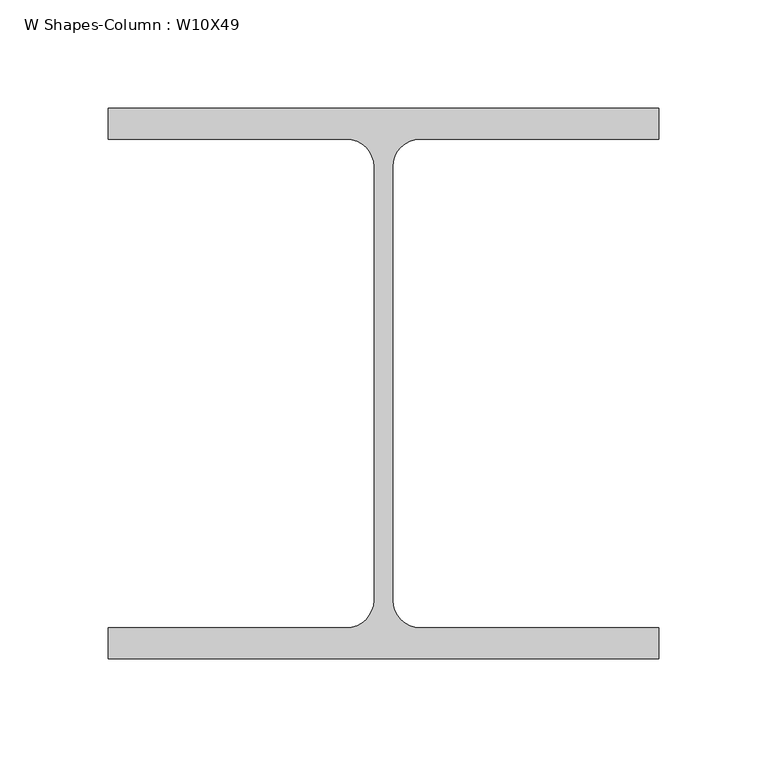
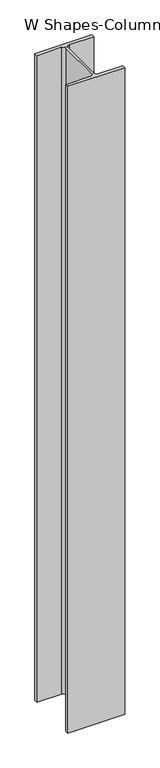
"""IFC4 building model written with IfcOpenShell, lengths in millimetres: column geometry, W Shapes-Column : W10X49."""

from ifc_helpers import new_model, si_unit, point, frame, frame_2d, origin, place, context, project, spatial, polyline, circle_curve, trimmed, segment, composite_curve, outline, extrude, source, transform, mapped, element, save


def w_shapes_column_w10x49_8035b166(model_context):
    return source(origin(), model_context, "Body", "SweptSolid", [
        extrude(outline(composite_curve([segment(polyline([(127.0, 127.0), (127.0, 112.776), (17.018, 112.776)]), True, "CONTINUOUS"), segment(trimmed(circle_curve(frame_2d((17.018, 100.076)), 12.7), [point((17.018, 112.776))], [point((4.318, 100.076))], True, "CARTESIAN"), True, "CONTINUOUS"), segment(polyline([(4.318, 100.076), (4.318, -100.076)]), True, "CONTINUOUS"), segment(trimmed(circle_curve(frame_2d((17.018, -100.076)), 12.7), [point((4.318, -100.076))], [point((17.018, -112.776))], True, "CARTESIAN"), True, "CONTINUOUS"), segment(polyline([(17.018, -112.776), (127.0, -112.776), (127.0, -127.0), (-127.0, -127.0), (-127.0, -112.776), (-17.018, -112.776)]), True, "CONTINUOUS"), segment(trimmed(circle_curve(frame_2d((-17.018, -100.076)), 12.7), [point((-17.018, -112.776))], [point((-4.318, -100.076))], True, "CARTESIAN"), True, "CONTINUOUS"), segment(polyline([(-4.318, -100.076), (-4.318, 100.076)]), True, "CONTINUOUS"), segment(trimmed(circle_curve(frame_2d((-17.018, 100.076)), 12.7), [point((-4.318, 100.076))], [point((-17.018, 112.776))], True, "CARTESIAN"), True, "CONTINUOUS"), segment(polyline([(-17.018, 112.776), (-127.0, 112.776), (-127.0, 127.0), (127.0, 127.0)]), True, "CONTINUOUS")], self_intersect=False)), frame((0.0, 0.0, 9144.0), z_axis=(0.0, 0.0, 1.0), x_axis=(1.0, 0.0, 0.0)), (0.0, 0.0, 1.0), 3048.0),
    ])


if __name__ == "__main__":
    model = new_model("IFC4")
    model_context = context("Model", 3, world=origin())
    ifc_project = project(units=[si_unit("LENGTHUNIT", "METRE", prefix="MILLI")], contexts=[model_context])
    site = spatial("IfcSite", under=ifc_project)
    building = spatial("IfcBuilding", under=site)
    placement = place(None, origin())
    w_shapes_column_w10x49_shape = w_shapes_column_w10x49_8035b166(model_context)
    element("IfcColumn", 1, ObjectType="W Shapes-Column : W10X49", at=placement, inside=building, context=model_context, shape_type="MappedRepresentation", body=[
        mapped(w_shapes_column_w10x49_shape, transform((0.0, 0.0, 0.0), x_axis=(1.0, 0.0, 0.0), y_axis=(0.0, 1.0, 0.0), z_axis=(0.0, 0.0, 1.0))),
    ])
    save(model, "model.ifc")

# Revit data of these elements
# Type "W Shapes-Column : W10X49"
#   Section Name Key = "W10x49"
#   Assembly Code = "B10"
#   Width = 10.000"
#   Web Thickness = 0.340"
#   Web Fillet = 0.500"
#   Warping Constant = 2070.00 in⁶
#   Torsional Moment of Inertia = 1.39 in⁴
#   Section Area = 14.40 in²
#   Plastic Modulus weak axis = 28.30 in³
#   Plastic Modulus strong axis = 60.40 in³
#   Perimeter = 58.50 ft²/ft
#   Nominal Weight = 49.00 lbf/ft
#   Moment of Inertia weak axis = 93.40 in⁴
#   Moment of Inertia strong axis = 272.00 in⁴
#   Height = 10.000"
#   Flange Thickness = 0.560"
#   Elastic Modulus weak axis = 18.70 in³
#   Elastic Modulus strong axis = 54.60 in³
#   Centroid Vertical = 5.000"
#   Centroid Horizontal = 5.000"
#   Bolt Spacing = 0' - 5 1/2"
#   Structural Material [instance default] = Steel ASTM A992
#   Principal Axes Angle = 0
# Element 1 (IfcColumn, "W Shapes-Column : W10X49")
#   Materials on its faces: "Steel ASTM A992"
# Materials
#   "Steel ASTM A992": class "Metal", colour RGB 199 199 199, transparency 0, Description = "Structural steel 50ksi", Cost = 0
